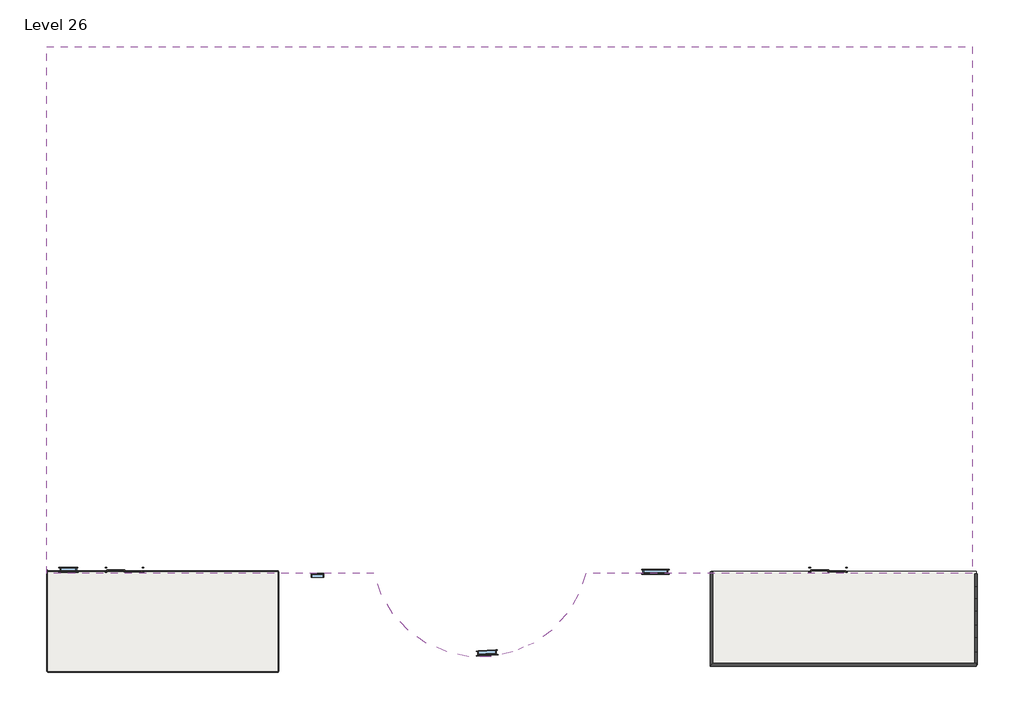
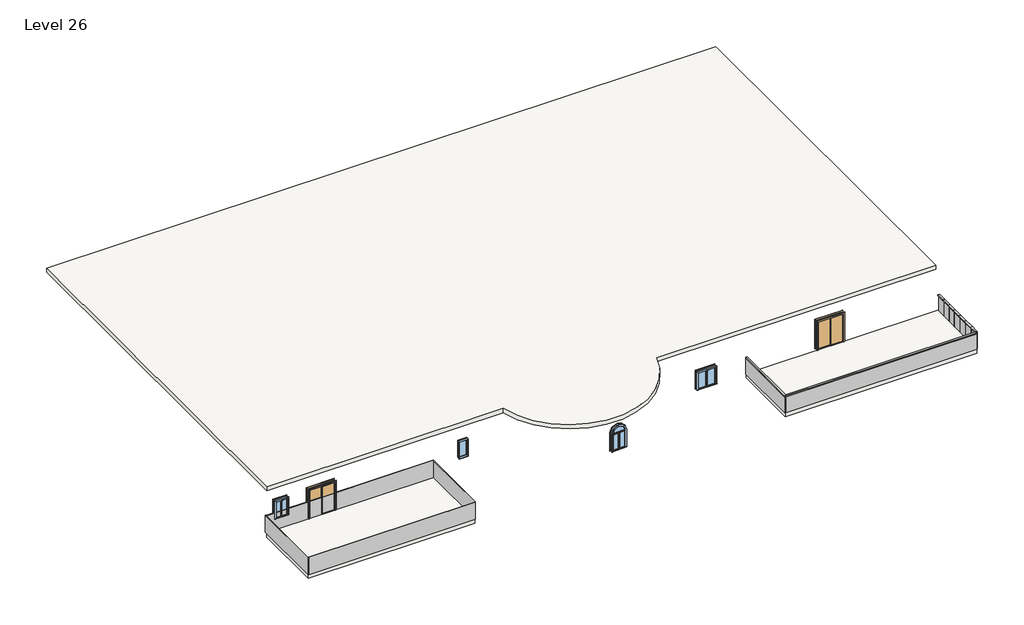
# One storey: 13 plates, 10 members, 4 windows, 3 slabs, 2 doors.
"""IFC4 building model written with IfcOpenShell, lengths in millimetres."""

from ifc_helpers import new_model, si_unit, point, frame, frame_2d, origin, place, context, project, spatial, polyline, circle_curve, trimmed, segment, composite_curve, outline, extrude, transform, mapped, element, save
from components import door_076b30e0, member_75074519, member_5e365d0c, member_6b5d0785, member_d3852687, member_6e28d7e1, member_c8189573, member_a84de01e, member_104e7e8d, system_panel_glazed_6a65e850, system_panel_glazed_188537b2, system_panel_glazed_c28eec11, system_panel_glazed_a1f4a93c, system_panel_glazed_73c284ea, system_panel_glazed_547c043f, system_panel_glazed_7e85febf, system_panel_glazed_ea481271, system_panel_glazed_53c2349a, system_panel_glazed_dfd0d0b7, window_cf4adaea, window_bb17773d, window_0862ab64, window_80bd9af0

model = new_model("IFC4")

# Units and contexts
model_context = context("Model", 3, world=origin())
ifc_project = project(units=[si_unit("LENGTHUNIT", "METRE", prefix="MILLI")], contexts=[model_context])

# Site, building, storey
site = spatial("IfcSite", under=ifc_project)
building = spatial("IfcBuilding", under=site)
storey = spatial("IfcBuildingStorey", under=building, Name="Level 26", Elevation=43281.6)

# Doors
placement = place(None, origin())
door_shape = door_076b30e0(model_context)
element("IfcDoor", 1, ObjectType="Door-Double-Sliding : 68\" x 80\"", at=placement, inside=storey, context=model_context, shape_type="MappedRepresentation", body=[
    mapped(door_shape, transform((-16064.585279, -12227.7237084, 43281.6), x_axis=(-1.0, 0.0, 0.0), y_axis=(0.0, -1.0, 0.0), z_axis=(0.0, 0.0, 1.0))),
])
element("IfcDoor", 2, ObjectType="Door-Double-Sliding : 68\" x 80\"", at=placement, inside=storey, context=model_context, shape_type="MappedRepresentation", body=[
    mapped(door_shape, transform((18377.814721, -12227.7237084, 43281.6), x_axis=(-1.0, 0.0, 0.0), y_axis=(0.0, -1.0, 0.0), z_axis=(0.0, 0.0, 1.0))),
])

# Members
member_shape = member_75074519(model_context)
element("IfcMember", 3, ObjectType="Rectangular Mullion : 2.5\" x 5\" rectangular", at=placement, inside=storey, context=model_context, shape_type="MappedRepresentation", body=[
    mapped(member_shape, transform((25621.5594464, -17004.2033949, 43281.6), x_axis=(0.0, -1.0, 0.0), y_axis=(-1.0, 0.0, 0.0), z_axis=(0.0, 0.0, -1.0))),
])
member_2_shape = member_5e365d0c(model_context)
element("IfcMember", 4, ObjectType="Rectangular Mullion : 2.5\" x 5\" rectangular", at=placement, inside=storey, context=model_context, shape_type="MappedRepresentation", body=[
    mapped(member_2_shape, transform((25621.5594464, -15683.4033949, 44500.8), x_axis=(0.0, 0.0, 1.0), y_axis=(-1.0, 0.0, 0.0), z_axis=(0.0, -1.0, 0.0))),
])
member_3_shape = member_6b5d0785(model_context)
element("IfcMember", 5, ObjectType="Rectangular Mullion : 2.5\" x 5\" rectangular", at=placement, inside=storey, context=model_context, shape_type="MappedRepresentation", body=[
    mapped(member_3_shape, transform((25621.5594464, -13167.9502705, 44500.8), x_axis=(0.0, 0.0, 1.0), y_axis=(-1.0, 0.0, 0.0), z_axis=(0.0, -1.0, 0.0))),
])
element("IfcMember", 6, ObjectType="Rectangular Mullion : 2.5\" x 5\" rectangular", at=placement, inside=storey, context=model_context, shape_type="MappedRepresentation", body=[
    mapped(member_3_shape, transform((25621.5594464, -13777.9768327, 44500.8), x_axis=(0.0, 0.0, 1.0), y_axis=(-1.0, 0.0, 0.0), z_axis=(0.0, -1.0, 0.0))),
])
element("IfcMember", 7, ObjectType="Rectangular Mullion : 2.5\" x 5\" rectangular", at=placement, inside=storey, context=model_context, shape_type="MappedRepresentation", body=[
    mapped(member_3_shape, transform((25621.5594464, -14388.0033949, 44500.8), x_axis=(0.0, 0.0, 1.0), y_axis=(-1.0, 0.0, 0.0), z_axis=(0.0, -1.0, 0.0))),
])
member_4_shape = member_d3852687(model_context)
element("IfcMember", 8, ObjectType="Rectangular Mullion : 2.5\" x 5\" rectangular", at=placement, inside=storey, context=model_context, shape_type="MappedRepresentation", body=[
    mapped(member_4_shape, transform((25621.5594464, -15048.4033949, 44500.8), x_axis=(0.0, 0.0, 1.0), y_axis=(-1.0, 0.0, 0.0), z_axis=(0.0, -1.0, 0.0))),
])
member_5_shape = member_6e28d7e1(model_context)
element("IfcMember", 9, ObjectType="Rectangular Mullion : 2.5\" x 5\" rectangular", at=placement, inside=storey, context=model_context, shape_type="MappedRepresentation", body=[
    mapped(member_5_shape, transform((25621.5594464, -16369.2033949, 44500.8), x_axis=(0.0, 0.0, 1.0), y_axis=(-1.0, 0.0, 0.0), z_axis=(0.0, -1.0, 0.0))),
])
member_6_shape = member_c8189573(model_context)
element("IfcMember", 10, ObjectType="Rectangular Mullion : 2.5\" x 5\" rectangular", at=placement, inside=storey, context=model_context, shape_type="MappedRepresentation", body=[
    mapped(member_6_shape, transform((25621.5594464, -16940.7033949, 44500.8), x_axis=(0.0, 0.0, 1.0), y_axis=(-1.0, 0.0, 0.0), z_axis=(0.0, -1.0, 0.0))),
])
member_7_shape = member_a84de01e(model_context)
element("IfcMember", 11, ObjectType="Rectangular Mullion : 2.5\" x 5\" rectangular", at=placement, inside=storey, context=model_context, shape_type="MappedRepresentation", body=[
    mapped(member_7_shape, transform((12667.5594464, -12456.3237084, 44500.8), x_axis=(0.0, 0.0, 1.0), y_axis=(1.0, 0.0, 0.0), z_axis=(0.0, 1.0, 0.0))),
])
member_8_shape = member_104e7e8d(model_context)
element("IfcMember", 12, ObjectType="Rectangular Mullion : 2.5\" x 5\" rectangular", at=placement, inside=storey, context=model_context, shape_type="MappedRepresentation", body=[
    mapped(member_8_shape, transform((12667.5594464, -17004.2033949, 44500.8), x_axis=(0.0, 0.0, 1.0), y_axis=(0.0, 1.0, 0.0), z_axis=(-1.0, 0.0, 0.0))),
])

# Plates
system_panel_glazed_shape = system_panel_glazed_6a65e850(model_context)
element("IfcPlate", 13, ObjectType="System Panel : Glazed", at=placement, inside=storey, context=model_context, shape_type="MappedRepresentation", body=[
    mapped(system_panel_glazed_shape, transform((25621.5594464, -15365.9033949, 43281.6), x_axis=(0.0, -1.0, 0.0), y_axis=(1.0, 0.0, 0.0), z_axis=(0.0, 0.0, 1.0))),
])
system_panel_glazed_2_shape = system_panel_glazed_188537b2(model_context)
element("IfcPlate", 14, ObjectType="System Panel : Glazed", at=placement, inside=storey, context=model_context, shape_type="MappedRepresentation", body=[
    mapped(system_panel_glazed_2_shape, transform((25621.5594464, -12862.9369895, 43281.6), x_axis=(0.0, -1.0, 0.0), y_axis=(1.0, 0.0, 0.0), z_axis=(0.0, 0.0, 1.0))),
])
element("IfcPlate", 15, ObjectType="System Panel : Glazed", at=placement, inside=storey, context=model_context, shape_type="MappedRepresentation", body=[
    mapped(system_panel_glazed_2_shape, transform((25621.5594464, -14082.9901138, 43281.6), x_axis=(0.0, -1.0, 0.0), y_axis=(1.0, 0.0, 0.0), z_axis=(0.0, 0.0, 1.0))),
])
element("IfcPlate", 16, ObjectType="System Panel : Glazed", at=placement, inside=storey, context=model_context, shape_type="MappedRepresentation", body=[
    mapped(system_panel_glazed_2_shape, transform((25621.5594464, -13472.9635516, 43281.6), x_axis=(0.0, -1.0, 0.0), y_axis=(1.0, 0.0, 0.0), z_axis=(0.0, 0.0, 1.0))),
])
system_panel_glazed_3_shape = system_panel_glazed_c28eec11(model_context)
element("IfcPlate", 17, ObjectType="System Panel : Glazed", at=placement, inside=storey, context=model_context, shape_type="MappedRepresentation", body=[
    mapped(system_panel_glazed_3_shape, transform((25621.5594464, -16654.9533949, 43281.6), x_axis=(0.0, -1.0, 0.0), y_axis=(1.0, 0.0, 0.0), z_axis=(0.0, 0.0, 1.0))),
])
system_panel_glazed_4_shape = system_panel_glazed_a1f4a93c(model_context)
element("IfcPlate", 18, ObjectType="System Panel : Glazed", at=placement, inside=storey, context=model_context, shape_type="MappedRepresentation", body=[
    mapped(system_panel_glazed_4_shape, transform((25621.5594464, -16026.3033949, 43281.6), x_axis=(0.0, -1.0, 0.0), y_axis=(1.0, 0.0, 0.0), z_axis=(0.0, 0.0, 1.0))),
])
system_panel_glazed_5_shape = system_panel_glazed_73c284ea(model_context)
element("IfcPlate", 19, ObjectType="System Panel : Glazed", at=placement, inside=storey, context=model_context, shape_type="MappedRepresentation", body=[
    mapped(system_panel_glazed_5_shape, transform((25621.5594464, -14718.2033949, 43281.6), x_axis=(0.0, -1.0, 0.0), y_axis=(1.0, 0.0, 0.0), z_axis=(0.0, 0.0, 1.0))),
])
system_panel_glazed_6_shape = system_panel_glazed_547c043f(model_context)
element("IfcPlate", 20, ObjectType="System Panel : Glazed", at=placement, inside=storey, context=model_context, shape_type="MappedRepresentation", body=[
    mapped(system_panel_glazed_6_shape, transform((19144.5594464, -17004.2033949, 43281.6), x_axis=(-1.0, 0.0, 0.0), y_axis=(0.0, -1.0, 0.0), z_axis=(0.0, 0.0, 1.0))),
])
system_panel_glazed_7_shape = system_panel_glazed_7e85febf(model_context)
element("IfcPlate", 21, ObjectType="System Panel : Glazed", at=placement, inside=storey, context=model_context, shape_type="MappedRepresentation", body=[
    mapped(system_panel_glazed_7_shape, transform((12667.5594464, -14730.2635516, 43281.6), x_axis=(0.0, 1.0, 0.0), y_axis=(-1.0, 0.0, 0.0), z_axis=(0.0, 0.0, 1.0))),
])
system_panel_glazed_8_shape = system_panel_glazed_ea481271(model_context)
element("IfcPlate", 22, ObjectType="System Panel : Glazed", at=placement, inside=storey, context=model_context, shape_type="MappedRepresentation", body=[
    mapped(system_panel_glazed_8_shape, transform((-14184.985279, -12456.3237084, 43281.6), x_axis=(1.0, 0.0, 0.0), y_axis=(0.0, 1.0, 0.0), z_axis=(0.0, 0.0, 1.0))),
])
element("IfcPlate", 23, ObjectType="System Panel : Glazed", at=placement, inside=storey, context=model_context, shape_type="MappedRepresentation", body=[
    mapped(system_panel_glazed_8_shape, transform((-14184.985279, -17333.1237084, 43281.6), x_axis=(-1.0, 0.0, 0.0), y_axis=(0.0, -1.0, 0.0), z_axis=(0.0, 0.0, 1.0))),
])
system_panel_glazed_9_shape = system_panel_glazed_53c2349a(model_context)
element("IfcPlate", 24, ObjectType="System Panel : Glazed", at=placement, inside=storey, context=model_context, shape_type="MappedRepresentation", body=[
    mapped(system_panel_glazed_9_shape, transform((-8546.185279, -14894.7237084, 43281.6), x_axis=(0.0, -1.0, 0.0), y_axis=(1.0, 0.0, 0.0), z_axis=(0.0, 0.0, 1.0))),
])
system_panel_glazed_10_shape = system_panel_glazed_dfd0d0b7(model_context)
element("IfcPlate", 25, ObjectType="System Panel : Glazed", at=placement, inside=storey, context=model_context, shape_type="MappedRepresentation", body=[
    mapped(system_panel_glazed_10_shape, transform((-19823.785279, -14843.9237084, 43281.6), x_axis=(0.0, 1.0, 0.0), y_axis=(-1.0, 0.0, 0.0), z_axis=(0.0, 0.0, 1.0))),
])

# Slabs
element("IfcSlab", 26, ObjectType="Generic - 12\"", at=placement, inside=storey, context=model_context, shape_type="SweptSolid", body=[
    extrude(outline(composite_curve([segment(polyline([(25439.014721, 13276.0523961), (25439.014721, -12530.3476039), (6520.7594464, -12530.3476039)]), True, "CONTINUOUS"), segment(trimmed(circle_curve(frame_2d((1334.414721, -11299.7145626)), 5330.3498284), [point((6520.7594464, -12530.3476039))], [point((-3851.9300045, -12530.3476039))], False, "CARTESIAN"), True, "CONTINUOUS"), segment(polyline([(-3851.9300045, -12530.3476039), (-19874.585279, -12530.3476039), (-19874.585279, 13276.0523961), (25439.014721, 13276.0523961)]), True, "CONTINUOUS")], self_intersect=False)), frame((0.0, 0.0, 46341.6732819), z_axis=(0.0, 0.0, 1.0), x_axis=(1.0, 0.0, 0.0)), (0.0, 0.0, 1.0), 304.8),
])
element("IfcSlab", 27, ObjectType="Generic - 12\"", at=placement, inside=storey, context=model_context, shape_type="SweptSolid", body=[
    extrude(outline(polyline([(25621.5594464, -12432.2033949), (25621.5594464, -17004.2033949), (12667.5594464, -17004.2033949), (12667.5594464, -12432.2033949), (25621.5594464, -12432.2033949)])), frame((0.0, 0.0, 42976.8), z_axis=(0.0, 0.0, 1.0), x_axis=(1.0, 0.0, 0.0)), (0.0, 0.0, 1.0), 304.8),
])
element("IfcSlab", 28, ObjectType="Generic - 12\"", at=placement, inside=storey, context=model_context, shape_type="SweptSolid", body=[
    extrude(outline(polyline([(-8546.185279, -12456.3237084), (-8546.185279, -17333.1237084), (-19823.785279, -17333.1237084), (-19823.785279, -12456.3237084), (-8546.185279, -12456.3237084)])), frame((0.0, 0.0, 42976.8), z_axis=(0.0, 0.0, 1.0), x_axis=(1.0, 0.0, 0.0)), (0.0, 0.0, 1.0), 304.8),
])

# Windows
window_shape = window_cf4adaea(model_context)
element("IfcWindow", 29, ObjectType="36\" x 48\"", at=placement, inside=storey, context=model_context, shape_type="MappedRepresentation", body=[
    mapped(window_shape, transform((1695.2692061, -16425.5670906, 43281.6), x_axis=(-0.9983172783942381, -0.0579880303124814, 0.0), y_axis=(0.0579880303124814, -0.9983172783942381, 0.0), z_axis=(0.0, 0.0, 1.0))),
])
window_2_shape = window_bb17773d(model_context)
element("IfcWindow", 30, ObjectType="Casement Dbl with Trim : 32\" x 48\"", at=placement, inside=storey, context=model_context, shape_type="MappedRepresentation", body=[
    mapped(window_2_shape, transform((-18807.785279, -12335.6737084, 43153.5858782), x_axis=(-1.0, 0.0, 0.0), y_axis=(0.0, -1.0, 0.0), z_axis=(0.0, 0.0, 1.0))),
])
window_3_shape = window_0862ab64(model_context)
element("IfcWindow", 31, ObjectType="Casement Dbl with Trim : 48\" x 48\"", at=placement, inside=storey, context=model_context, shape_type="MappedRepresentation", body=[
    mapped(window_3_shape, transform((9924.3594464, -12437.2737084, 42460.1672913), x_axis=(-1.0, 0.0, 0.0), y_axis=(0.0, -1.0, 0.0), z_axis=(0.0, 0.0, 1.0))),
])
window_4_shape = window_80bd9af0(model_context)
element("IfcWindow", 32, ObjectType="Fixed : 24\" x 48\"", at=placement, inside=storey, context=model_context, shape_type="MappedRepresentation", body=[
    mapped(window_4_shape, transform((-6577.685279, -12617.2007309, 43281.6), x_axis=(1.0, 0.0, 0.0), y_axis=(0.0, 1.0, 0.0), z_axis=(0.0, 0.0, 1.0))),
])

save(model, "model.ifc")

# Revit data of these elements
# Type "Door-Double-Sliding : 68\" x 80\""
#   Type Mark = "10"
#   Construction Type Id = "opn-d45"
#   Assembly Code = "C1020"
#   Analytic Construction = "Wood frame, double glass door "
#   Thickness = 0' - 2"
#   Thermal Resistance (R) = 1.8150 (h·ft²·°F)/BTU
#   Heat Transfer Coefficient (U) = 0.5510 BTU/(h·ft²·°F)
#   Height = 6' - 8"
#   Rail Width = 0' - 2"
#   Stiles = 0' - 2"
#   Trim Projection Ext = 0' - 1"
#   Trim Projection Int = 0' - 1"
#   Trim Width = 0' - 3"
#   Width = 5' - 8"
#   Define Thermal Properties by = 1
#   Glazing = Glass
#   Panel Material = Wood - Birch - Solid Stained Light Low Gloss
#   Trim Material = Paint - Sienna
#   Visual Light Transmittance = 0
#   Solar Heat Gain Coefficient = 0
#   Function = (empty or 0)
#   Wall Closure = (empty or 0)
# Type "Rectangular Mullion : 2.5\" x 5\" rectangular"
#   built-in parameter 1007304 = 0.416667 (stored number, unit not read)
#   built-in parameter 1007301 = 0.104167 (stored number, unit not read)
#   built-in parameter 1007300 = 0.104167 (stored number, unit not read)
# Type "System Panel : Glazed"
#   Construction Type Id = "GSP4R"
#   Analytic Construction = "1/8 in Pilkington single glazing"
#   Visual Light Transmittance = 0.9
#   Solar Heat Gain Coefficient = 0.86
#   Heat Transfer Coefficient (U) = 1.18115 BTU/(h·ft²·°F)
# Type "Generic - 12\""
#   Assembly Code = "B1010"
#   Function = 0
#   Layers, outside or top first: 1' - 0" no material (function 1)
# Type "36\" x 48\""
#   Type Mark = "38"
#   Construction Type Id = "SGL"
#   Assembly Code = "B2020100"
#   Analytic Construction = "Large single-glazed windows"
#   Visual Light Transmittance = 0.9
#   Solar Heat Gain Coefficient = 0.86
#   Heat Transfer Coefficient (U) = 0.979472 BTU/(h·ft²·°F)
#   Height = 4' - 0"
#   Default Sill Height = 3' - 0"
#   Trim Projection - Ext. = 0' - 0 1/2"
#   Trim Projection - Int. = 0' - 0 3/4"
#   Trim Width - Exterior = 0' - 3 1/2"
#   Trim Width - Interior = 0' - 3 1/2"
#   Width = 3' - 0"
#   Window Inset = 0' - 0 3/4"
#   Define Thermal Properties by = 1
#   Glass Pane Material = Glass
#   Sash Material = Sash
#   Trim Exterior Material = Trim
#   Trim Interior Material = Trim
#   Wall Closure = (empty or 0)
# Type "Casement Dbl with Trim : 32\" x 48\""
#   Type Mark = "36"
#   Construction Type Id = "GSP4R"
#   Assembly Code = "B2020100"
#   Analytic Construction = "1/8 in Pilkington single glazing"
#   Visual Light Transmittance = 0.9
#   Solar Heat Gain Coefficient = 0.78
#   Heat Transfer Coefficient (U) = 0.6496 BTU/(h·ft²·°F)
#   Height = 4' - 0"
#   Default Sill Height = 3' - 0"
#   Trim Projection - Ext. = 0' - 0 1/2"
#   Trim Projection - Int. = 0' - 0 3/4"
#   Trim Width - Exterior = 0' - 3 1/2"
#   Trim Width - Interior = 0' - 3 1/2"
#   Width = 2' - 8"
#   Window Inset = 0' - 0 3/4"
#   Define Thermal Properties by = 1
#   Glass Pane Material = Glass
#   Sash Material = Sash
#   Trim Exterior Material = Trim
#   Trim Interior Material = Trim
#   Wall Closure = (empty or 0)
# Type "Casement Dbl with Trim : 48\" x 48\""
#   Type Mark = "34"
#   Construction Type Id = "GSP4R"
#   Assembly Code = "B2020100"
#   Analytic Construction = "1/8 in Pilkington single glazing"
#   Visual Light Transmittance = 0.9
#   Solar Heat Gain Coefficient = 0.78
#   Heat Transfer Coefficient (U) = 0.6496 BTU/(h·ft²·°F)
#   Height = 4' - 0"
#   Default Sill Height = 3' - 0"
#   Trim Projection - Ext. = 0' - 0 1/2"
#   Trim Projection - Int. = 0' - 0 3/4"
#   Trim Width - Exterior = 0' - 3 1/2"
#   Trim Width - Interior = 0' - 3 1/2"
#   Width = 4' - 0"
#   Window Inset = 0' - 0 3/4"
#   Define Thermal Properties by = 1
#   Glass Pane Material = Glass
#   Sash Material = Sash
#   Trim Exterior Material = Trim
#   Trim Interior Material = Trim
#   Wall Closure = (empty or 0)
# Type "Fixed : 24\" x 48\""
#   Type Mark = "2"
#   Construction Type Id = "GSP4R"
#   Assembly Code = "B2020100"
#   Analytic Construction = "1/8 in Pilkington single glazing"
#   Visual Light Transmittance = 0.9
#   Solar Heat Gain Coefficient = 0.78
#   Heat Transfer Coefficient (U) = 0.6496 BTU/(h·ft²·°F)
#   Height = 4' - 0"
#   Default Sill Height = 3' - 0"
#   Width = 2' - 0"
#   Window Inset = 0' - 0 3/4"
#   Define Thermal Properties by = 1
#   Glass Pane Material = Glass
#   Sash Material = Sash
#   Wall Closure = (empty or 0)
# Elements 1, 2 (IfcDoor, "Door-Double-Sliding : 68\" x 80\"")
#   Phase Created = New Construction
#   Materials on its faces: "Paint - Sienna", "Wood - Birch - Solid Stained Light Low Gloss", "Glass"
# Elements 3, 4, 5, 6, 7, 8, 9, 10, 11, 12 (IfcMember, "Rectangular Mullion : 2.5\" x 5\" rectangular")
#   Phase Created = New Construction
#   Materials on its faces: "Aluminum"
# Elements 13, 14, 15, 16, 17, 18, 19, 20, 21, 22, 23, 24, 25 (IfcPlate, "System Panel : Glazed")
#   Phase Created = New Construction
#   Materials on its faces: "Glass"
# Element 26 (IfcSlab, "Generic - 12\"")
#   Height Offset From Level = 11' - 0.47533"
#   Phase Created = New Construction
#   Materials on its faces: "Default Floor"
# Elements 27, 28 (IfcSlab, "Generic - 12\"")
#   Height Offset From Level = 0' - 0"
#   Phase Created = New Construction
#   Materials on its faces: "Default Floor"
# Element 29 (IfcWindow, "36\" x 48\"")
#   Mark = "21"
#   Phase Created = New Construction
#   Materials on its faces: "Sash", "Trim", "Glass"
# Element 30 (IfcWindow, "Casement Dbl with Trim : 32\" x 48\"")
#   Mark = "38"
#   Phase Created = New Construction
#   Materials on its faces: "Sash", "Trim", "Glass"
# Element 31 (IfcWindow, "Casement Dbl with Trim : 48\" x 48\"")
#   Mark = "4"
#   Phase Created = New Construction
#   Materials on its faces: "Sash", "Trim", "Glass"
# Element 32 (IfcWindow, "Fixed : 24\" x 48\"")
#   Mark = "72"
#   Phase Created = New Construction
#   Materials on its faces: "Sash", "Glass"
# Materials
#   "Glass": class "Glass", colour RGB 0 128 192, transparency 0.75, Description = "Soda Lime Glass", Cost = 0
#   "Wood - Birch - Solid Stained Light Low Gloss": class "Wood", colour RGB 210 159 95, transparency 0, Cost = 0
#   "Paint - Sienna": colour RGB 118 70 51, transparency 0, Cost = 0
#   "Sash": class "Wood", colour RGB 224 178 126, transparency 0
#   "Trim": class "Wood", colour RGB 224 178 126, transparency 0
#   "Aluminum": class "Metal", colour RGB 247 247 247, transparency 0, Description = "Aluminum 6061", Cost = 0
#   "Default Floor": colour RGB 128 128 128, transparency 0
